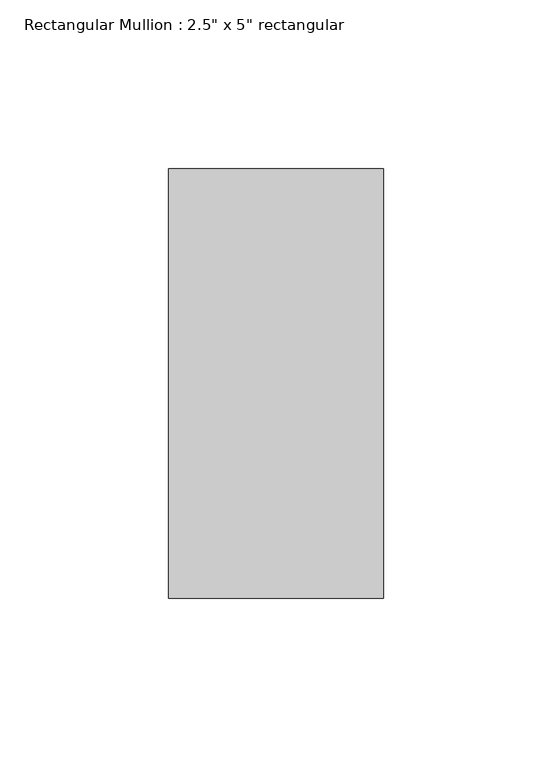
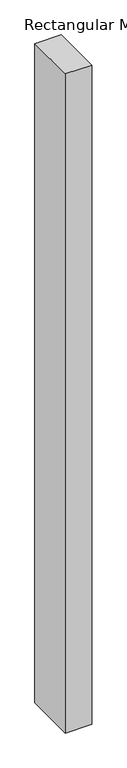
"""IFC4 building model written with IfcOpenShell, lengths in millimetres: member geometry."""

from ifc_helpers import new_model, si_unit, frame, origin, place, context, project, spatial, polyline, outline, extrude, source, transform, mapped, element, save


def member_67d70a96(model_context):
    return source(origin(), model_context, "Body", "SweptSolid", [
        extrude(outline(polyline([(0.0, 63.5), (0.0, -63.5), (-63.5, -63.5), (-63.5, 63.5), (0.0, 63.5)])), frame((0.0, 0.0, -1680.4980219), z_axis=(0.0, 0.0, 1.0), x_axis=(1.0, 0.0, 0.0)), (0.0, 0.0, 1.0), 1680.4980219),
    ])


if __name__ == "__main__":
    model = new_model("IFC4")
    model_context = context("Model", 3, world=origin())
    ifc_project = project(units=[si_unit("LENGTHUNIT", "METRE", prefix="MILLI")], contexts=[model_context])
    site = spatial("IfcSite", under=ifc_project)
    building = spatial("IfcBuilding", under=site)
    placement = place(None, origin())
    member_shape = member_67d70a96(model_context)
    element("IfcMember", 1, ObjectType="Rectangular Mullion : 2.5\" x 5\" rectangular", at=placement, inside=building, context=model_context, shape_type="MappedRepresentation", body=[
        mapped(member_shape, transform((0.0, 0.0, 0.0), x_axis=(1.0, 0.0, 0.0), y_axis=(0.0, 1.0, 0.0), z_axis=(0.0, 0.0, 1.0))),
    ])
    save(model, "model.ifc")

# Revit data of these elements
# Type "Rectangular Mullion : 2.5\" x 5\" rectangular"
#   built-in parameter 1007304 = 0.416667 (stored number, unit not read)
#   built-in parameter 1007301 = 0.104167 (stored number, unit not read)
#   built-in parameter 1007300 = 0.104167 (stored number, unit not read)
# Element 1 (IfcMember, "Rectangular Mullion : 2.5\" x 5\" rectangular")
#   Materials on its faces: "Aluminum"
# Materials
#   "Aluminum": class "Metal", colour RGB 247 247 247, transparency 0, Description = "Aluminum 6061", Cost = 0
